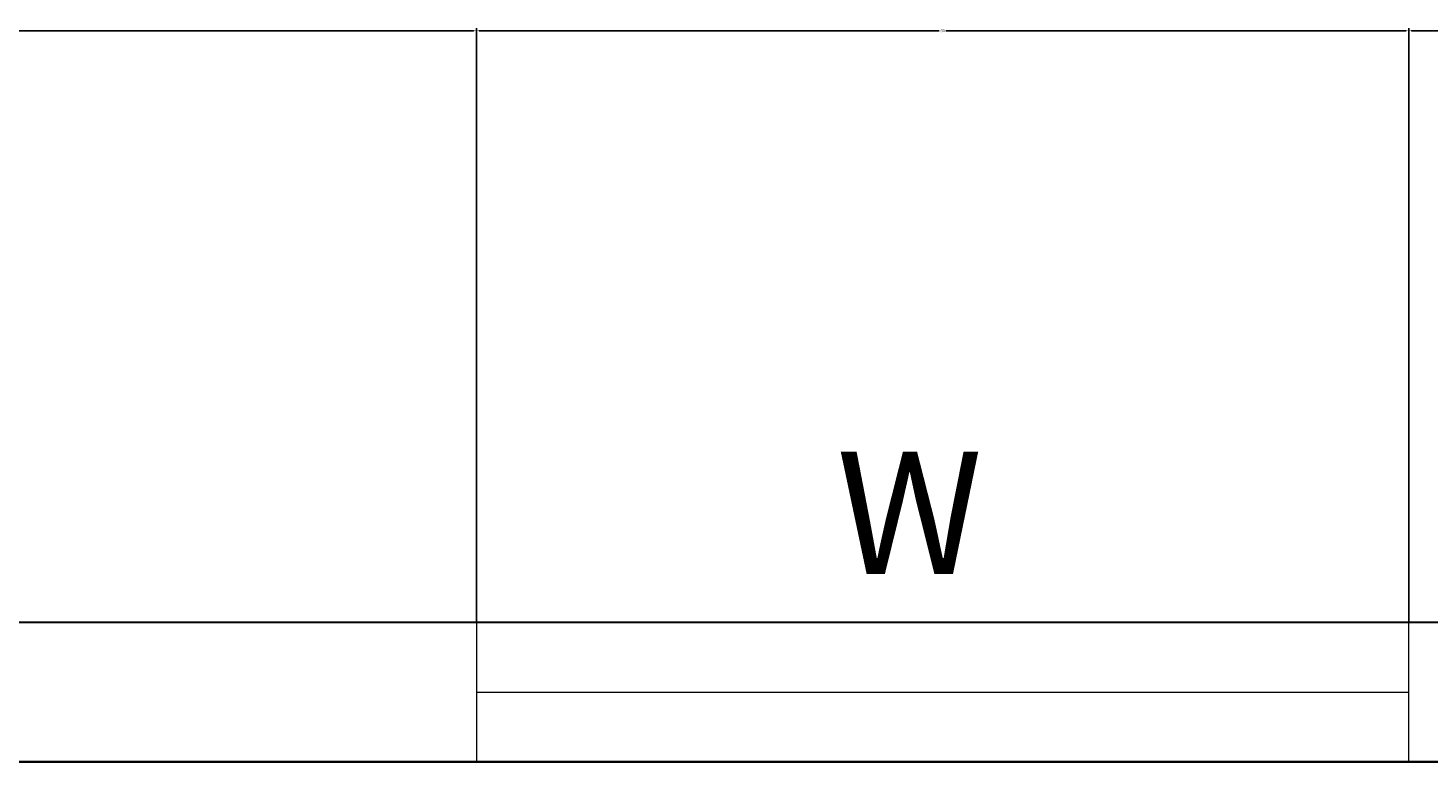
# Model space of a CAD drawing. Units: feet. Extents: x 2219 to 3039, y 1768 to 2369.
# Tile 11 of 16: x 2694 to 2784, y 2322 to 2369. Entities that reach past the tile are written whole.
import ezdxf

# ---------------------------------------------------------------- set-up
doc = ezdxf.new("R2010")
doc.units = ezdxf.units.FT
for name, color, linetype, lineweight in [('A-ANNO-DIMS', 2, 'Continuous', 18), ('A-ANNO-TEXT', 7, 'Continuous', 18), ('A-GLAZ', 4, 'Continuous', 18), ('A-WALL', 7, 'Continuous', 35), ('C-PROP', 7, 'Continuous', 30)]:
    doc.layers.add(name, color=color, linetype=linetype, lineweight=lineweight)
doc.styles.get("Standard").update_dxf_attribs({"font": 'arial.ttf'})
doc.dimstyles.get("Standard").update_dxf_attribs({"dimtxt": 0.18, "dimasz": 0.18, "dimexe": 0.18, "dimexo": 0.0625, "dimgap": 0.09, "dimtad": 0, "dimtih": 1, "dimtoh": 1, "dimdec": 4, "dimzin": 0, "dimdsep": 46, "dimtxsty": 'Standard', "dimcen": 0.09, "dimadec": 0, "dimazin": 0, "dimtfac": 1, "dimtdec": 4, "dimtofl": 0, "dimtmove": 0, "dimatfit": 3, "dimfxl": 1, "dimtolj": 1, "dimtzin": 0, "dimarcsym": 0})

# ---------------------------------------------------------------- blocks, each defined once
blk = doc.blocks.new('*D55')
at = {"layer": 'A-ANNO-DIMS', "color": 0, "lineweight": -2, "transparency": 16777216}
for p, q in [((2400.382, 2330.985), (2400.382, 2369.153)), ((2400.562, 2368.973), (2561.103, 2368.973)), ((2722.22, 2368.973), (2561.679, 2368.973)), ((2722.4, 2330.985), (2722.4, 2369.153))]:
    blk.add_line(p, q, dxfattribs=at)
at = {"layer": 'A-ANNO-DIMS', "color": 0, "transparency": 16777216}
for points in [[(2400.562, 2369.003), (2400.562, 2368.943), (2400.382, 2368.973)], [(2722.22, 2369.003), (2722.22, 2368.943), (2722.4, 2368.973)]]:
    blk.add_solid(points, dxfattribs=at)
at = {"layer": 'Defpoints', "color": 0, "transparency": 16777216}
for p in [(2722.4, 2368.973), (2400.382, 2330.923), (2722.4, 2330.923)]:
    blk.add_point(p, dxfattribs=at)
at = {"layer": 'A-ANNO-DIMS', "color": 0, "transparency": 16777216, "insert": (2561.391, 2368.973), "char_height": 0.18, "attachment_point": 5}
blk.add_mtext('\\A1;322', dxfattribs=at)
blk = doc.blocks.new('*D56')
at = {"layer": 'A-ANNO-DIMS', "color": 0, "lineweight": -2, "transparency": 16777216}
for p, q in [((2722.4, 2330.985), (2722.4, 2369.153)), ((2722.58, 2368.973), (2752.18, 2368.973)), ((2782.22, 2368.973), (2752.619, 2368.973)), ((2782.4, 2330.985), (2782.4, 2369.153))]:
    blk.add_line(p, q, dxfattribs=at)
at = {"layer": 'A-ANNO-DIMS', "color": 0, "transparency": 16777216}
for points in [[(2722.58, 2369.003), (2722.58, 2368.943), (2722.4, 2368.973)], [(2782.22, 2369.003), (2782.22, 2368.943), (2782.4, 2368.973)]]:
    blk.add_solid(points, dxfattribs=at)
at = {"layer": 'Defpoints', "color": 0, "transparency": 16777216}
for p in [(2782.4, 2368.973), (2722.4, 2330.923), (2782.4, 2330.923)]:
    blk.add_point(p, dxfattribs=at)
at = {"layer": 'A-ANNO-DIMS', "color": 0, "transparency": 16777216, "insert": (2752.4, 2368.973), "char_height": 0.18, "attachment_point": 5}
blk.add_mtext('\\A1;60', dxfattribs=at)
blk = doc.blocks.new('*D57')
at = {"layer": 'A-ANNO-DIMS', "color": 0, "lineweight": -2, "transparency": 16777216}
for p, q in [((2782.4, 2330.985), (2782.4, 2369.153)), ((2782.58, 2368.973), (2837.637, 2368.973)), ((2893.22, 2368.973), (2838.163, 2368.973)), ((2893.4, 2330.985), (2893.4, 2369.153))]:
    blk.add_line(p, q, dxfattribs=at)
at = {"layer": 'A-ANNO-DIMS', "color": 0, "transparency": 16777216}
for points in [[(2782.58, 2369.003), (2782.58, 2368.943), (2782.4, 2368.973)], [(2893.22, 2369.003), (2893.22, 2368.943), (2893.4, 2368.973)]]:
    blk.add_solid(points, dxfattribs=at)
at = {"layer": 'Defpoints', "color": 0, "transparency": 16777216}
for p in [(2893.4, 2368.973), (2782.4, 2330.923), (2893.4, 2330.923)]:
    blk.add_point(p, dxfattribs=at)
at = {"layer": 'A-ANNO-DIMS', "color": 0, "transparency": 16777216, "insert": (2837.9, 2368.973), "char_height": 0.18, "attachment_point": 5}
blk.add_mtext('\\A1;111', dxfattribs=at)

msp = doc.modelspace()

# ---------------------------------------------------------------- linework, layer by layer
at = {"layer": 'A-GLAZ'}
for p, q in [((2722.4, 2330.923), (2722.4, 2321.923)), ((2782.4, 2321.923), (2782.4, 2330.923)), ((2722.4, 2326.423), (2782.4, 2326.423))]:
    msp.add_line(p, q, dxfattribs=at)
at = {"layer": 'A-WALL'}
msp.add_line((2610.4, 2321.923), (2834.4, 2321.923), dxfattribs=at)
at = {"layer": 'C-PROP'}
msp.add_line((2314.4, 2330.923), (3000.4, 2330.923), dxfattribs=at)

# ---------------------------------------------------------------- texts
at = {"layer": 'A-ANNO-TEXT'}
msp.add_text('W', height=7.858, dxfattribs=at).set_placement((2745.569, 2334.03))

# ---------------------------------------------------------------- dimensions: what is measured, and where the dimension line sits
at = {"layer": 'A-ANNO-DIMS'}
for base, p1, p2, picture, middle in [((2722.4, 2368.973), (2400.382, 2330.923), (2722.4, 2330.923), '*D55', (2561.391, 2368.973)), ((2782.4, 2368.973), (2722.4, 2330.923), (2782.4, 2330.923), '*D56', (2752.4, 2368.973)), ((2893.4, 2368.973), (2782.4, 2330.923), (2893.4, 2330.923), '*D57', (2837.9, 2368.973))]:
    dim = msp.add_linear_dim(base=base, p1=p1, p2=p2, dimstyle='Standard', override={"dimdec": 0, "dimlfac": 1, "dimrnd": 0, "dimzin": 0, "dimdsep": 46, "dimlunit": 2}, dxfattribs=at)
    dim.commit()
    dim.dimension.update_dxf_attribs({"geometry": picture, "text_midpoint": middle})

doc.saveas('drawing.dxf')
